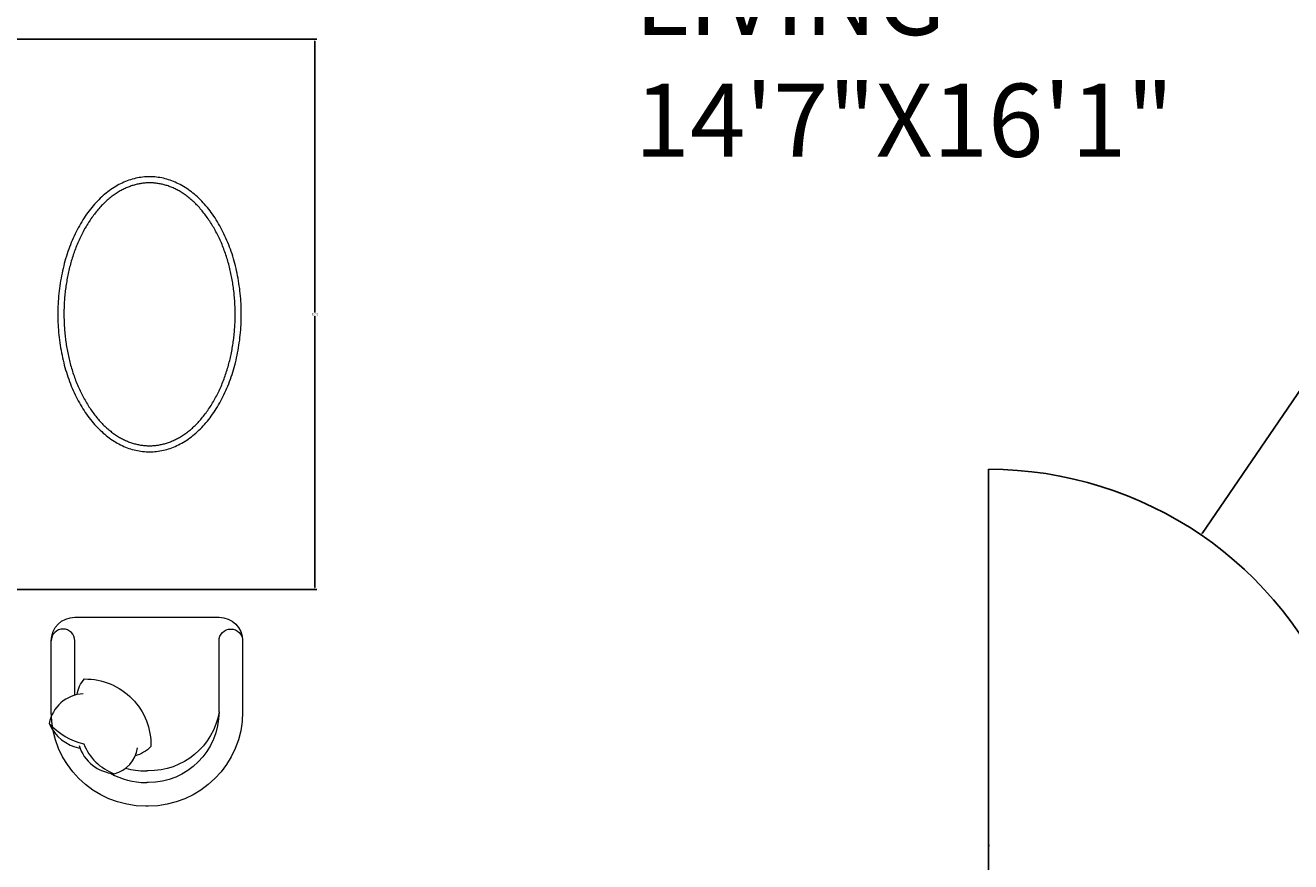
# Model space of a CAD drawing. Units: inches. Extents: x 1676 to 2199, y 1657 to 2783.
# Tile 3 of 10: x 1786 to 1907, y 1905 to 1985. Entities that reach past the tile are written whole.
import ezdxf

# ---------------------------------------------------------------- set-up
doc = ezdxf.new("R2010")
doc.units = ezdxf.units.IN
for name, color, linetype, lineweight in [('A-ANNO-DIMS', 2, 'Continuous', 18), ('A-AREA-IDEN', 7, 'Continuous', 18), ('A-DOOR', 4, 'Continuous', 25), ('A-FURN', 8, 'Continuous', 13)]:
    doc.layers.add(name, color=color, linetype=linetype, lineweight=lineweight)
doc.styles.get("Standard").update_dxf_attribs({"font": 'arial.ttf'})
doc.dimstyles.get("Standard").update_dxf_attribs({"dimtxt": 0.18, "dimasz": 0.18, "dimexe": 0.18, "dimexo": 0.0625, "dimgap": 0.09, "dimtad": 0, "dimtih": 1, "dimtoh": 1, "dimdec": 4, "dimzin": 0, "dimdsep": 46, "dimtxsty": 'Standard', "dimcen": 0.09, "dimadec": 0, "dimazin": 0, "dimtfac": 1, "dimtdec": 4, "dimtofl": 0, "dimtmove": 0, "dimatfit": 3, "dimfxl": 1, "dimtolj": 1, "dimtzin": 0, "dimarcsym": 0})

# ---------------------------------------------------------------- blocks, each defined once
blk = doc.blocks.new('*D56')
at = {"layer": 'A-ANNO-DIMS', "color": 0, "lineweight": -2, "transparency": 16777216}
for p, q in [((1781.71, 1983.79), (1813.98, 1983.79)), ((1813.8, 1983.61), (1813.8, 1957.62)), ((1813.8, 1931.26), (1813.8, 1957.25)), ((1781.71, 1931.08), (1813.98, 1931.08))]:
    blk.add_line(p, q, dxfattribs=at)
at = {"layer": 'A-ANNO-DIMS', "color": 0, "transparency": 16777216}
for points in [[(1813.77, 1983.61), (1813.83, 1983.61), (1813.8, 1983.79)], [(1813.77, 1931.26), (1813.83, 1931.26), (1813.8, 1931.08)]]:
    blk.add_solid(points, dxfattribs=at)
at = {"layer": 'Defpoints', "color": 0, "transparency": 16777216}
for p in [(1781.65, 1983.79), (1781.65, 1931.08), (1813.8, 1931.08)]:
    blk.add_point(p, dxfattribs=at)
at = {"layer": 'A-ANNO-DIMS', "color": 0, "transparency": 16777216, "insert": (1813.8, 1957.43), "char_height": 0.18, "attachment_point": 5}
blk.add_mtext('\\A1;52.72', dxfattribs=at)
blk = doc.blocks.new('*D81')
at = {"layer": 'A-ANNO-DIMS', "color": 0, "lineweight": -2, "transparency": 16777216}
for p, q in [((1910.86, 1954.14), (1898.76, 1936.45)), ((1911.04, 1954.14), (1910.86, 1954.14)), ((1878.23, 1906.55), (1878.41, 1906.55)), ((1878.32, 1906.46), (1878.32, 1906.64))]:
    blk.add_line(p, q, dxfattribs=at)
at = {"layer": 'A-ANNO-DIMS', "color": 0, "transparency": 16777216}
blk.add_solid([(1898.73, 1936.46), (1898.78, 1936.43), (1898.66, 1936.3)], dxfattribs=at)
at = {"layer": 'Defpoints', "color": 0, "transparency": 16777216}
for p in [(1898.66, 1936.3), (1878.32, 1906.55)]:
    blk.add_point(p, dxfattribs=at)
at = {"layer": 'A-ANNO-DIMS', "color": 0, "transparency": 16777216, "insert": (1911.59, 1954.14), "char_height": 0.18, "attachment_point": 5}
blk.add_mtext('\\A1;R36.034', dxfattribs=at)

msp = doc.modelspace()

# ---------------------------------------------------------------- linework, layer by layer
at = {"layer": 'A-DOOR'}
msp.add_line((1878.3163, 1894.5871), (1878.3163, 1942.5871), dxfattribs=at)
msp.add_arc((1878.3163, 1906.5528), 36.0343, 21.266188, 90, dxfattribs=at)
at = {"layer": 'A-FURN', "ltscale": 0.03}
msp.add_lwpolyline([(1797.7122, 1928.4136), (1804.6154, 1928.4136, -0.41421356), (1806.8787, 1926.1503), (1806.8787, 1919.3603, -0.41421356), (1797.8254, 1910.307), (1797.7122, 1910.307), (1797.5991, 1910.307, -0.41421356), (1788.5457, 1919.3603), (1788.5457, 1926.1503, -0.41421356), (1790.8091, 1928.4136), (1797.7122, 1928.4136)], format="xyb", dxfattribs=at)
at = {"layer": 'A-FURN'}
for points in [[(1790.8091, 1920.947), (1790.8091, 1926.1503, 0.41421356), (1789.6774, 1927.282), (1789.6774, 1927.282, 0.41421356), (1788.5457, 1926.1503)], [(1804.6154, 1919.3602), (1804.6154, 1926.1503, -0.41421356), (1805.7471, 1927.282), (1805.7471, 1927.282, -0.41421356), (1806.8787, 1926.1503)], [(1791.0329, 1921.0014, -0.16554063), (1791.733, 1922.4967, -0.42598917), (1798.0887, 1916.0137, -0.12152332), (1796.58, 1915.1202, 7.11546429)], [(1791.6033, 1921.0704, 0.35677236), (1788.3606, 1918.2179, 0.24954205), (1791.2988, 1915.8672, -9.61688035)], [(1804.6154, 1919.3603, -0.37271891), (1797.8254, 1913.702), (1797.7122, 1913.702)], [(1804.6154, 1919.3603, -0.41421356), (1797.8254, 1912.5703), (1797.7122, 1912.5703)], [(1788.3606, 1918.2179, 0.14772988), (1791.6682, 1916.273, 0.21334276), (1794.5866, 1913.4205, 0.17866181)], [(1791.2112, 1916.118, 0.30666349), (1794.5866, 1913.4205, 0.30632997), (1796.7916, 1915.8841, -0.87284716)], [(1795.6696, 1913.9458, 0.07238424), (1797.5991, 1913.702), (1797.7122, 1913.702)], [(1794.2286, 1913.4659, 0.13059149), (1797.5991, 1912.5703), (1797.7122, 1912.5703)]]:
    msp.add_lwpolyline(points, format="xyb", dxfattribs=at)
at = {"layer": 'A-FURN', "ltscale": 0.03}
msp.add_polyline3d([(1797.9632, 1970.6124, 0), (1797.797, 1970.61, 0), (1797.6308, 1970.603, 0), (1797.4647, 1970.5912, 0), (1797.2988, 1970.5746, 0), (1797.1331, 1970.5534, 0), (1796.9677, 1970.5275, 0), (1796.8027, 1970.4969, 0), (1796.6381, 1970.4616, 0), (1796.474, 1970.4217, 0), (1796.3104, 1970.3771, 0), (1796.1474, 1970.3278, 0), (1795.9851, 1970.274, 0), (1795.8234, 1970.2155, 0), (1795.6625, 1970.1525, 0), (1795.5025, 1970.0849, 0), (1795.3433, 1970.0128, 0), (1795.1851, 1969.9362, 0), (1795.0279, 1969.8551, 0), (1794.8717, 1969.7695, 0), (1794.7166, 1969.6796, 0), (1794.5627, 1969.5852, 0), (1794.41, 1969.4865, 0), (1794.2586, 1969.3835, 0), (1794.1085, 1969.2762, 0), (1793.9597, 1969.1646, 0), (1793.8125, 1969.0489, 0), (1793.6667, 1968.929, 0), (1793.5224, 1968.805, 0), (1793.3797, 1968.6769, 0), (1793.2387, 1968.5448, 0), (1793.0994, 1968.4087, 0), (1792.9618, 1968.2686, 0), (1792.826, 1968.1247, 0), (1792.692, 1967.977, 0), (1792.56, 1967.8255, 0), (1792.4298, 1967.6702, 0), (1792.3017, 1967.5113, 0), (1792.1755, 1967.3488, 0), (1792.0515, 1967.1827, 0), (1791.9296, 1967.0132, 0), (1791.8098, 1966.8402, 0), (1791.6922, 1966.6638, 0), (1791.5769, 1966.4842, 0), (1791.4638, 1966.3013, 0), (1791.3531, 1966.1152, 0), (1791.2448, 1965.926, 0), (1791.1389, 1965.7337, 0), (1791.0354, 1965.5385, 0), (1790.9343, 1965.3404, 0), (1790.8359, 1965.1395, 0), (1790.7399, 1964.9358, 0), (1790.6466, 1964.7294, 0), (1790.5558, 1964.5204, 0), (1790.4677, 1964.3089, 0), (1790.3823, 1964.0949, 0), (1790.2997, 1963.8785, 0), (1790.2197, 1963.6598, 0), (1790.1426, 1963.4389, 0), (1790.0682, 1963.2158, 0), (1789.9967, 1962.9906, 0), (1789.928, 1962.7635, 0), (1789.8622, 1962.5345, 0), (1789.7993, 1962.3036, 0), (1789.7393, 1962.071, 0), (1789.6823, 1961.8367, 0), (1789.6282, 1961.6008, 0), (1789.5771, 1961.3635, 0), (1789.529, 1961.1247, 0), (1789.484, 1960.8847, 0), (1789.442, 1960.6434, 0), (1789.403, 1960.4009, 0), (1789.3671, 1960.1574, 0), (1789.3343, 1959.9129, 0), (1789.3045, 1959.6675, 0), (1789.2779, 1959.4213, 0), (1789.2544, 1959.1744, 0), (1789.234, 1958.9269, 0), (1789.2167, 1958.6788, 0), (1789.2026, 1958.4303, 0), (1789.1916, 1958.1815, 0), (1789.1837, 1957.9323, 0), (1789.179, 1957.683, 0), (1789.1774, 1957.4336, 0), (1789.179, 1957.1842, 0), (1789.1837, 1956.9349, 0), (1789.1916, 1956.6858, 0), (1789.2026, 1956.4369, 0), (1789.2167, 1956.1884, 0), (1789.234, 1955.9404, 0), (1789.2544, 1955.6928, 0), (1789.2779, 1955.4459, 0), (1789.3045, 1955.1998, 0), (1789.3343, 1954.9544, 0), (1789.3671, 1954.7099, 0), (1789.403, 1954.4663, 0), (1789.442, 1954.2239, 0), (1789.484, 1953.9826, 0), (1789.529, 1953.7425, 0), (1789.5771, 1953.5037, 0), (1789.6282, 1953.2664, 0), (1789.6823, 1953.0305, 0), (1789.7393, 1952.7963, 0), (1789.7993, 1952.5636, 0), (1789.8622, 1952.3328, 0), (1789.928, 1952.1037, 0), (1789.9967, 1951.8766, 0), (1790.0682, 1951.6514, 0), (1790.1426, 1951.4284, 0), (1790.2197, 1951.2074, 0), (1790.2997, 1950.9888, 0), (1790.3823, 1950.7724, 0), (1790.4677, 1950.5584, 0), (1790.5558, 1950.3468, 0), (1790.6466, 1950.1378, 0), (1790.7399, 1949.9314, 0), (1790.8359, 1949.7277, 0), (1790.9343, 1949.5268, 0), (1791.0354, 1949.3287, 0), (1791.1389, 1949.1335, 0), (1791.2448, 1948.9413, 0), (1791.3531, 1948.7521, 0), (1791.4638, 1948.566, 0), (1791.5769, 1948.3831, 0), (1791.6922, 1948.2034, 0), (1791.8098, 1948.0271, 0), (1791.9296, 1947.8541, 0), (1792.0515, 1947.6845, 0), (1792.1755, 1947.5184, 0), (1792.3017, 1947.3559, 0), (1792.4298, 1947.197, 0), (1792.56, 1947.0418, 0), (1792.692, 1946.8903, 0), (1792.826, 1946.7425, 0), (1792.9618, 1946.5986, 0), (1793.0994, 1946.4586, 0), (1793.2387, 1946.3225, 0), (1793.3797, 1946.1904, 0), (1793.5224, 1946.0623, 0), (1793.6667, 1945.9382, 0), (1793.8125, 1945.8183, 0), (1793.9597, 1945.7026, 0), (1794.1085, 1945.591, 0), (1794.2586, 1945.4837, 0), (1794.41, 1945.3807, 0), (1794.5627, 1945.282, 0), (1794.7166, 1945.1877, 0), (1794.8717, 1945.0977, 0), (1795.0279, 1945.0122, 0), (1795.1851, 1944.9311, 0), (1795.3433, 1944.8544, 0), (1795.5025, 1944.7823, 0), (1795.6625, 1944.7147, 0), (1795.8234, 1944.6517, 0), (1795.9851, 1944.5932, 0), (1796.1474, 1944.5394, 0), (1796.3104, 1944.4902, 0), (1796.474, 1944.4456, 0), (1796.6381, 1944.4056, 0), (1796.8027, 1944.3703, 0), (1796.9677, 1944.3397, 0), (1797.1331, 1944.3138, 0), (1797.2988, 1944.2926, 0), (1797.4647, 1944.2761, 0), (1797.6308, 1944.2643, 0), (1797.797, 1944.2572, 0), (1797.9632, 1944.2548, 0), (1798.1295, 1944.2572, 0), (1798.2957, 1944.2643, 0), (1798.4618, 1944.2761, 0), (1798.6277, 1944.2926, 0), (1798.7934, 1944.3138, 0), (1798.9588, 1944.3397, 0), (1799.1238, 1944.3703, 0), (1799.2884, 1944.4056, 0), (1799.4525, 1944.4456, 0), (1799.6161, 1944.4902, 0), (1799.7791, 1944.5394, 0), (1799.9414, 1944.5932, 0), (1800.1031, 1944.6517, 0), (1800.2639, 1944.7147, 0), (1800.424, 1944.7823, 0), (1800.5832, 1944.8544, 0), (1800.7414, 1944.9311, 0), (1800.8986, 1945.0122, 0), (1801.0548, 1945.0977, 0), (1801.2099, 1945.1877, 0), (1801.3638, 1945.282, 0), (1801.5165, 1945.3807, 0), (1801.6679, 1945.4837, 0), (1801.818, 1945.591, 0), (1801.9667, 1945.7026, 0), (1802.114, 1945.8183, 0), (1802.2598, 1945.9382, 0), (1802.4041, 1946.0623, 0), (1802.5467, 1946.1904, 0), (1802.6878, 1946.3225, 0), (1802.8271, 1946.4586, 0), (1802.9647, 1946.5986, 0), (1803.1005, 1946.7425, 0), (1803.2345, 1946.8903, 0), (1803.3665, 1947.0418, 0), (1803.4967, 1947.197, 0), (1803.6248, 1947.3559, 0), (1803.7509, 1947.5184, 0), (1803.875, 1947.6845, 0), (1803.9969, 1947.8541, 0), (1804.1167, 1948.0271, 0), (1804.2343, 1948.2034, 0), (1804.3496, 1948.3831, 0), (1804.4627, 1948.566, 0), (1804.5734, 1948.7521, 0), (1804.6817, 1948.9413, 0), (1804.7876, 1949.1335, 0), (1804.8911, 1949.3287, 0), (1804.9921, 1949.5268, 0), (1805.0906, 1949.7277, 0), (1805.1866, 1949.9314, 0), (1805.2799, 1950.1378, 0), (1805.3707, 1950.3468, 0), (1805.4588, 1950.5584, 0), (1805.5442, 1950.7724, 0), (1805.6268, 1950.9888, 0), (1805.7068, 1951.2074, 0), (1805.7839, 1951.4284, 0), (1805.8583, 1951.6514, 0), (1805.9298, 1951.8766, 0), (1805.9985, 1952.1037, 0), (1806.0643, 1952.3328, 0), (1806.1272, 1952.5636, 0), (1806.1872, 1952.7963, 0), (1806.2442, 1953.0305, 0), (1806.2983, 1953.2664, 0), (1806.3494, 1953.5037, 0), (1806.3975, 1953.7425, 0), (1806.4425, 1953.9826, 0), (1806.4845, 1954.2239, 0), (1806.5235, 1954.4663, 0), (1806.5594, 1954.7099, 0), (1806.5922, 1954.9544, 0), (1806.622, 1955.1998, 0), (1806.6486, 1955.4459, 0), (1806.6721, 1955.6928, 0), (1806.6925, 1955.9404, 0), (1806.7098, 1956.1884, 0), (1806.7239, 1956.4369, 0), (1806.7349, 1956.6858, 0), (1806.7428, 1956.9349, 0), (1806.7475, 1957.1842, 0), (1806.7491, 1957.4336, 0), (1806.7475, 1957.683, 0), (1806.7428, 1957.9323, 0), (1806.7349, 1958.1815, 0), (1806.7239, 1958.4303, 0), (1806.7098, 1958.6788, 0), (1806.6925, 1958.9269, 0), (1806.6721, 1959.1744, 0), (1806.6486, 1959.4213, 0), (1806.622, 1959.6675, 0), (1806.5922, 1959.9129, 0), (1806.5594, 1960.1574, 0), (1806.5235, 1960.4009, 0), (1806.4845, 1960.6434, 0), (1806.4425, 1960.8847, 0), (1806.3975, 1961.1247, 0), (1806.3494, 1961.3635, 0), (1806.2983, 1961.6008, 0), (1806.2442, 1961.8367, 0), (1806.1872, 1962.071, 0), (1806.1272, 1962.3036, 0), (1806.0643, 1962.5345, 0), (1805.9985, 1962.7635, 0), (1805.9298, 1962.9906, 0), (1805.8583, 1963.2158, 0), (1805.7839, 1963.4389, 0), (1805.7068, 1963.6598, 0), (1805.6268, 1963.8785, 0), (1805.5442, 1964.0949, 0), (1805.4588, 1964.3089, 0), (1805.3707, 1964.5204, 0), (1805.2799, 1964.7294, 0), (1805.1866, 1964.9358, 0), (1805.0906, 1965.1395, 0), (1804.9921, 1965.3404, 0), (1804.8911, 1965.5385, 0), (1804.7876, 1965.7337, 0), (1804.6817, 1965.926, 0), (1804.5734, 1966.1152, 0), (1804.4627, 1966.3013, 0), (1804.3496, 1966.4842, 0), (1804.2343, 1966.6638, 0), (1804.1167, 1966.8402, 0), (1803.9969, 1967.0132, 0), (1803.875, 1967.1827, 0), (1803.7509, 1967.3488, 0), (1803.6248, 1967.5113, 0), (1803.4967, 1967.6702, 0), (1803.3665, 1967.8255, 0), (1803.2345, 1967.977, 0), (1803.1005, 1968.1247, 0), (1802.9647, 1968.2686, 0), (1802.8271, 1968.4087, 0), (1802.6878, 1968.5448, 0), (1802.5467, 1968.6769, 0), (1802.4041, 1968.805, 0), (1802.2598, 1968.929, 0), (1802.114, 1969.0489, 0), (1801.9667, 1969.1646, 0), (1801.818, 1969.2762, 0), (1801.6679, 1969.3835, 0), (1801.5165, 1969.4865, 0), (1801.3638, 1969.5852, 0), (1801.2099, 1969.6796, 0), (1801.0548, 1969.7695, 0), (1800.8986, 1969.8551, 0), (1800.7414, 1969.9362, 0), (1800.5832, 1970.0128, 0), (1800.424, 1970.0849, 0), (1800.2639, 1970.1525, 0), (1800.1031, 1970.2155, 0), (1799.9414, 1970.274, 0), (1799.7791, 1970.3278, 0), (1799.6161, 1970.3771, 0), (1799.4525, 1970.4217, 0), (1799.2884, 1970.4616, 0), (1799.1238, 1970.4969, 0), (1798.9588, 1970.5275, 0), (1798.7934, 1970.5534, 0), (1798.6277, 1970.5746, 0), (1798.4618, 1970.5912, 0), (1798.2957, 1970.603, 0), (1798.1295, 1970.61, 0), (1797.9632, 1970.6124, 0)], dxfattribs=at)
at = {"layer": 'A-FURN'}
msp.add_polyline3d([(1797.9632, 1970.0267, 0), (1797.8734, 1970.0259, 0), (1797.7831, 1970.0236, 0), (1797.6925, 1970.0197, 0), (1797.6014, 1970.0142, 0), (1797.51, 1970.0071, 0), (1797.4182, 1969.9984, 0), (1797.326, 1969.9881, 0), (1797.2335, 1969.976, 0), (1797.1407, 1969.9623, 0), (1797.0476, 1969.9469, 0), (1796.9541, 1969.9297, 0), (1796.8604, 1969.9108, 0), (1796.7664, 1969.8901, 0), (1796.6721, 1969.8676, 0), (1796.5776, 1969.8433, 0), (1796.4829, 1969.8172, 0), (1796.3879, 1969.7892, 0), (1796.2927, 1969.7594, 0), (1796.1973, 1969.7276, 0), (1796.1017, 1969.6939, 0), (1796.0059, 1969.6583, 0), (1795.91, 1969.6208, 0), (1795.814, 1969.5812, 0), (1795.7179, 1969.5396, 0), (1795.6217, 1969.4961, 0), (1795.5255, 1969.4506, 0), (1795.4293, 1969.403, 0), (1795.3331, 1969.3535, 0), (1795.2369, 1969.3019, 0), (1795.1409, 1969.2484, 0), (1795.0449, 1969.1928, 0), (1794.9491, 1969.1352, 0), (1794.8535, 1969.0756, 0), (1794.758, 1969.014, 0), (1794.6628, 1968.9503, 0), (1794.5678, 1968.8847, 0), (1794.4732, 1968.817, 0), (1794.3788, 1968.7473, 0), (1794.2847, 1968.6755, 0), (1794.1911, 1968.6017, 0), (1794.0978, 1968.5259, 0), (1794.005, 1968.448, 0), (1793.9126, 1968.3679, 0), (1793.8206, 1968.2856, 0), (1793.7292, 1968.2012, 0), (1793.6383, 1968.1146, 0), (1793.5479, 1968.026, 0), (1793.4581, 1967.9352, 0), (1793.3688, 1967.8425, 0), (1793.2802, 1967.7477, 0), (1793.1923, 1967.651, 0), (1793.1049, 1967.5524, 0), (1793.0183, 1967.4518, 0), (1792.9324, 1967.3493, 0), (1792.8472, 1967.245, 0), (1792.7628, 1967.1389, 0), (1792.6791, 1967.031, 0), (1792.5963, 1966.9213, 0), (1792.5143, 1966.8099, 0), (1792.4331, 1966.6968, 0), (1792.3528, 1966.582, 0), (1792.2735, 1966.4656, 0), (1792.195, 1966.3476, 0), (1792.1175, 1966.228, 0), (1792.041, 1966.1069, 0), (1791.9655, 1965.9843, 0), (1791.8909, 1965.8601, 0), (1791.8175, 1965.7346, 0), (1791.7451, 1965.6076, 0), (1791.6738, 1965.4792, 0), (1791.6036, 1965.3494, 0), (1791.5346, 1965.2184, 0), (1791.4667, 1965.086, 0), (1791.4, 1964.9523, 0), (1791.3345, 1964.8175, 0), (1791.2703, 1964.6814, 0), (1791.2073, 1964.5441, 0), (1791.1456, 1964.4057, 0), (1791.0853, 1964.2662, 0), (1791.0262, 1964.1256, 0), (1790.9686, 1963.9839, 0), (1790.9123, 1963.8412, 0), (1790.8574, 1963.6976, 0), (1790.8039, 1963.5531, 0), (1790.7518, 1963.4082, 0), (1790.7012, 1963.263, 0), (1790.652, 1963.1173, 0), (1790.6041, 1962.9713, 0), (1790.5577, 1962.8249, 0), (1790.5126, 1962.6782, 0), (1790.469, 1962.5311, 0), (1790.4267, 1962.3837, 0), (1790.3858, 1962.2359, 0), (1790.3462, 1962.0879, 0), (1790.308, 1961.9395, 0), (1790.2712, 1961.7908, 0), (1790.2356, 1961.6419, 0), (1790.2015, 1961.4926, 0), (1790.1686, 1961.3431, 0), (1790.1371, 1961.1934, 0), (1790.107, 1961.0434, 0), (1790.0781, 1960.8932, 0), (1790.0505, 1960.7427, 0), (1790.0243, 1960.592, 0), (1789.9993, 1960.4411, 0), (1789.9756, 1960.2901, 0), (1789.9533, 1960.1388, 0), (1789.9322, 1959.9873, 0), (1789.9123, 1959.8357, 0), (1789.8938, 1959.684, 0), (1789.8765, 1959.532, 0), (1789.8604, 1959.38, 0), (1789.8456, 1959.2278, 0), (1789.832, 1959.0755, 0), (1789.8197, 1958.9231, 0), (1789.8086, 1958.7706, 0), (1789.7988, 1958.618, 0), (1789.7901, 1958.4654, 0), (1789.7827, 1958.3126, 0), (1789.7764, 1958.1598, 0), (1789.7714, 1958.007, 0), (1789.7676, 1957.8541, 0), (1789.7649, 1957.7012, 0), (1789.7635, 1957.5483, 0), (1789.7632, 1957.3954, 0), (1789.764, 1957.2425, 0), (1789.7661, 1957.0896, 0), (1789.7693, 1956.9367, 0), (1789.7738, 1956.7838, 0), (1789.7794, 1956.631, 0), (1789.7862, 1956.4782, 0), (1789.7943, 1956.3255, 0), (1789.8035, 1956.1729, 0), (1789.814, 1956.0204, 0), (1789.8257, 1955.8679, 0), (1789.8387, 1955.7156, 0), (1789.8529, 1955.5633, 0), (1789.8683, 1955.4112, 0), (1789.885, 1955.2592, 0), (1789.9029, 1955.1074, 0), (1789.9221, 1954.9557, 0), (1789.9426, 1954.8042, 0), (1789.9643, 1954.6528, 0), (1789.9873, 1954.5016, 0), (1790.0116, 1954.3506, 0), (1790.0372, 1954.1999, 0), (1790.0641, 1954.0493, 0), (1790.0924, 1953.8989, 0), (1790.1219, 1953.7488, 0), (1790.1527, 1953.5989, 0), (1790.1849, 1953.4493, 0), (1790.2184, 1953.2999, 0), (1790.2532, 1953.1509, 0), (1790.2894, 1953.002, 0), (1790.3269, 1952.8535, 0), (1790.3658, 1952.7053, 0), (1790.4061, 1952.5574, 0), (1790.4477, 1952.4098, 0), (1790.4906, 1952.2625, 0), (1790.535, 1952.1156, 0), (1790.5807, 1951.9691, 0), (1790.6279, 1951.8229, 0), (1790.6764, 1951.677, 0), (1790.7263, 1951.5316, 0), (1790.7777, 1951.3865, 0), (1790.8304, 1951.2419, 0), (1790.8846, 1951.0977, 0), (1790.9402, 1950.9545, 0), (1790.9972, 1950.8124, 0), (1791.0556, 1950.6712, 0), (1791.1153, 1950.5312, 0), (1791.1763, 1950.3922, 0), (1791.2387, 1950.2544, 0), (1791.3023, 1950.1177, 0), (1791.3671, 1949.9822, 0), (1791.4332, 1949.8479, 0), (1791.5005, 1949.7149, 0), (1791.5689, 1949.5832, 0), (1791.6386, 1949.4528, 0), (1791.7093, 1949.3237, 0), (1791.7811, 1949.196, 0), (1791.8541, 1949.0697, 0), (1791.9281, 1948.9449, 0), (1792.0031, 1948.8215, 0), (1792.0791, 1948.6996, 0), (1792.1561, 1948.5792, 0), (1792.2341, 1948.4604, 0), (1792.313, 1948.3432, 0), (1792.3929, 1948.2276, 0), (1792.4736, 1948.1137, 0), (1792.5552, 1948.0014, 0), (1792.6376, 1947.8909, 0), (1792.7209, 1947.7821, 0), (1792.8049, 1947.6751, 0), (1792.8897, 1947.5698, 0), (1792.9753, 1947.4665, 0), (1793.0615, 1947.3649, 0), (1793.1485, 1947.2653, 0), (1793.2362, 1947.1676, 0), (1793.3245, 1947.0719, 0), (1793.4134, 1946.9781, 0), (1793.5029, 1946.8864, 0), (1793.593, 1946.7967, 0), (1793.6837, 1946.7091, 0), (1793.7748, 1946.6236, 0), (1793.8665, 1946.5402, 0), (1793.9587, 1946.4591, 0), (1794.0513, 1946.3801, 0), (1794.1444, 1946.3032, 0), (1794.2379, 1946.2284, 0), (1794.3317, 1946.1556, 0), (1794.4259, 1946.0849, 0), (1794.5205, 1946.0162, 0), (1794.6153, 1945.9495, 0), (1794.7104, 1945.8848, 0), (1794.8057, 1945.8222, 0), (1794.9013, 1945.7616, 0), (1794.997, 1945.703, 0), (1795.0929, 1945.6464, 0), (1795.1889, 1945.5918, 0), (1795.285, 1945.5393, 0), (1795.3812, 1945.4887, 0), (1795.4774, 1945.4402, 0), (1795.5736, 1945.3937, 0), (1795.6698, 1945.3491, 0), (1795.7659, 1945.3066, 0), (1795.862, 1945.266, 0), (1795.958, 1945.2274, 0), (1796.0538, 1945.1909, 0), (1796.1495, 1945.1562, 0), (1796.245, 1945.1235, 0), (1796.3403, 1945.0927, 0), (1796.4354, 1945.0638, 0), (1796.5303, 1945.0368, 0), (1796.6249, 1945.0115, 0), (1796.7193, 1944.9882, 0), (1796.8134, 1944.9666, 0), (1796.9073, 1944.9468, 0), (1797.0009, 1944.9287, 0), (1797.0942, 1944.9124, 0), (1797.1871, 1944.8979, 0), (1797.2798, 1944.885, 0), (1797.3721, 1944.8738, 0), (1797.4641, 1944.8642, 0), (1797.5557, 1944.8564, 0), (1797.647, 1944.8501, 0), (1797.7378, 1944.8454, 0), (1797.8283, 1944.8423, 0), (1797.9184, 1944.8408, 0), (1798.0081, 1944.8408, 0), (1798.0982, 1944.8423, 0), (1798.1887, 1944.8454, 0), (1798.2795, 1944.8501, 0), (1798.3708, 1944.8564, 0), (1798.4624, 1944.8642, 0), (1798.5544, 1944.8738, 0), (1798.6467, 1944.885, 0), (1798.7393, 1944.8979, 0), (1798.8323, 1944.9124, 0), (1798.9256, 1944.9287, 0), (1799.0192, 1944.9468, 0), (1799.1131, 1944.9666, 0), (1799.2072, 1944.9882, 0), (1799.3016, 1945.0115, 0), (1799.3962, 1945.0368, 0), (1799.4911, 1945.0638, 0), (1799.5862, 1945.0927, 0), (1799.6815, 1945.1235, 0), (1799.777, 1945.1562, 0), (1799.8727, 1945.1909, 0), (1799.9685, 1945.2274, 0), (1800.0645, 1945.266, 0), (1800.1605, 1945.3066, 0), (1800.2567, 1945.3491, 0), (1800.3529, 1945.3937, 0), (1800.4491, 1945.4402, 0), (1800.5453, 1945.4887, 0), (1800.6415, 1945.5393, 0), (1800.7376, 1945.5918, 0), (1800.8336, 1945.6464, 0), (1800.9295, 1945.703, 0), (1801.0252, 1945.7616, 0), (1801.1208, 1945.8222, 0), (1801.2161, 1945.8848, 0), (1801.3112, 1945.9495, 0), (1801.406, 1946.0162, 0), (1801.5006, 1946.0849, 0), (1801.5948, 1946.1556, 0), (1801.6886, 1946.2284, 0), (1801.7821, 1946.3032, 0), (1801.8752, 1946.3801, 0), (1801.9678, 1946.4591, 0), (1802.06, 1946.5402, 0), (1802.1516, 1946.6236, 0), (1802.2428, 1946.7091, 0), (1802.3335, 1946.7967, 0), (1802.4236, 1946.8864, 0), (1802.5131, 1946.9781, 0), (1802.602, 1947.0719, 0), (1802.6903, 1947.1676, 0), (1802.778, 1947.2653, 0), (1802.865, 1947.3649, 0), (1802.9512, 1947.4665, 0), (1803.0368, 1947.5698, 0), (1803.1216, 1947.6751, 0), (1803.2056, 1947.7821, 0), (1803.2889, 1947.8909, 0), (1803.3713, 1948.0014, 0), (1803.4529, 1948.1137, 0), (1803.5336, 1948.2276, 0), (1803.6135, 1948.3432, 0), (1803.6924, 1948.4604, 0), (1803.7704, 1948.5792, 0), (1803.8474, 1948.6996, 0), (1803.9234, 1948.8215, 0), (1803.9984, 1948.9449, 0), (1804.0724, 1949.0697, 0), (1804.1453, 1949.196, 0), (1804.2172, 1949.3237, 0), (1804.2879, 1949.4528, 0), (1804.3576, 1949.5832, 0), (1804.426, 1949.7149, 0), (1804.4933, 1949.8479, 0), (1804.5594, 1949.9822, 0), (1804.6242, 1950.1177, 0), (1804.6878, 1950.2544, 0), (1804.7502, 1950.3922, 0), (1804.8112, 1950.5312, 0), (1804.8709, 1950.6712, 0), (1804.9293, 1950.8124, 0), (1804.9863, 1950.9545, 0), (1805.0419, 1951.0977, 0), (1805.096, 1951.2419, 0), (1805.1488, 1951.3865, 0), (1805.2001, 1951.5316, 0), (1805.2501, 1951.677, 0), (1805.2986, 1951.8229, 0), (1805.3458, 1951.9691, 0), (1805.3915, 1952.1156, 0), (1805.4359, 1952.2625, 0), (1805.4788, 1952.4098, 0), (1805.5204, 1952.5574, 0), (1805.5607, 1952.7053, 0), (1805.5996, 1952.8535, 0), (1805.6371, 1953.002, 0), (1805.6733, 1953.1509, 0), (1805.7081, 1953.2999, 0), (1805.7416, 1953.4493, 0), (1805.7738, 1953.5989, 0), (1805.8046, 1953.7488, 0), (1805.8341, 1953.8989, 0), (1805.8623, 1954.0493, 0), (1805.8893, 1954.1999, 0), (1805.9149, 1954.3506, 0), (1805.9392, 1954.5016, 0), (1805.9622, 1954.6528, 0), (1805.9839, 1954.8042, 0), (1806.0044, 1954.9557, 0), (1806.0236, 1955.1074, 0), (1806.0415, 1955.2592, 0), (1806.0582, 1955.4112, 0), (1806.0736, 1955.5633, 0), (1806.0878, 1955.7156, 0), (1806.1008, 1955.8679, 0), (1806.1125, 1956.0204, 0), (1806.1229, 1956.1729, 0), (1806.1322, 1956.3255, 0), (1806.1403, 1956.4782, 0), (1806.1471, 1956.631, 0), (1806.1527, 1956.7838, 0), (1806.1572, 1956.9367, 0), (1806.1604, 1957.0896, 0), (1806.1625, 1957.2425, 0), (1806.1633, 1957.3954, 0), (1806.163, 1957.5483, 0), (1806.1616, 1957.7012, 0), (1806.1589, 1957.8541, 0), (1806.1551, 1958.007, 0), (1806.1501, 1958.1598, 0), (1806.1438, 1958.3126, 0), (1806.1364, 1958.4654, 0), (1806.1277, 1958.618, 0), (1806.1179, 1958.7706, 0), (1806.1068, 1958.9231, 0), (1806.0944, 1959.0755, 0), (1806.0809, 1959.2278, 0), (1806.0661, 1959.38, 0), (1806.05, 1959.532, 0), (1806.0327, 1959.684, 0), (1806.0142, 1959.8357, 0), (1805.9943, 1959.9873, 0), (1805.9732, 1960.1388, 0), (1805.9508, 1960.2901, 0), (1805.9272, 1960.4411, 0), (1805.9022, 1960.592, 0), (1805.876, 1960.7427, 0), (1805.8484, 1960.8932, 0), (1805.8195, 1961.0434, 0), (1805.7894, 1961.1934, 0), (1805.7578, 1961.3431, 0), (1805.725, 1961.4926, 0), (1805.6908, 1961.6419, 0), (1805.6553, 1961.7908, 0), (1805.6185, 1961.9395, 0), (1805.5803, 1962.0879, 0), (1805.5407, 1962.2359, 0), (1805.4998, 1962.3837, 0), (1805.4575, 1962.5311, 0), (1805.4138, 1962.6782, 0), (1805.3688, 1962.8249, 0), (1805.3224, 1962.9713, 0), (1805.2745, 1963.1173, 0), (1805.2253, 1963.263, 0), (1805.1747, 1963.4082, 0), (1805.1226, 1963.5531, 0), (1805.0691, 1963.6976, 0), (1805.0142, 1963.8412, 0), (1804.9579, 1963.9839, 0), (1804.9003, 1964.1256, 0), (1804.8412, 1964.2662, 0), (1804.7808, 1964.4057, 0), (1804.7192, 1964.5441, 0), (1804.6562, 1964.6814, 0), (1804.592, 1964.8175, 0), (1804.5265, 1964.9523, 0), (1804.4598, 1965.086, 0), (1804.3919, 1965.2184, 0), (1804.3229, 1965.3494, 0), (1804.2527, 1965.4792, 0), (1804.1814, 1965.6076, 0), (1804.109, 1965.7346, 0), (1804.0356, 1965.8601, 0), (1803.961, 1965.9843, 0), (1803.8855, 1966.1069, 0), (1803.809, 1966.228, 0), (1803.7315, 1966.3476, 0), (1803.653, 1966.4656, 0), (1803.5736, 1966.582, 0), (1803.4934, 1966.6968, 0), (1803.4122, 1966.8099, 0), (1803.3302, 1966.9213, 0), (1803.2474, 1967.031, 0), (1803.1637, 1967.1389, 0), (1803.0793, 1967.245, 0), (1802.9941, 1967.3493, 0), (1802.9082, 1967.4518, 0), (1802.8216, 1967.5524, 0), (1802.7342, 1967.651, 0), (1802.6463, 1967.7477, 0), (1802.5576, 1967.8425, 0), (1802.4684, 1967.9352, 0), (1802.3786, 1968.026, 0), (1802.2882, 1968.1146, 0), (1802.1973, 1968.2012, 0), (1802.1059, 1968.2856, 0), (1802.0139, 1968.3679, 0), (1801.9215, 1968.448, 0), (1801.8287, 1968.5259, 0), (1801.7354, 1968.6017, 0), (1801.6417, 1968.6755, 0), (1801.5477, 1968.7473, 0), (1801.4533, 1968.817, 0), (1801.3586, 1968.8847, 0), (1801.2637, 1968.9503, 0), (1801.1685, 1969.014, 0), (1801.073, 1969.0756, 0), (1800.9774, 1969.1352, 0), (1800.8816, 1969.1928, 0), (1800.7856, 1969.2484, 0), (1800.6896, 1969.3019, 0), (1800.5934, 1969.3535, 0), (1800.4972, 1969.403, 0), (1800.401, 1969.4506, 0), (1800.3048, 1969.4961, 0), (1800.2086, 1969.5396, 0), (1800.1125, 1969.5812, 0), (1800.0165, 1969.6208, 0), (1799.9206, 1969.6583, 0), (1799.8248, 1969.6939, 0), (1799.7292, 1969.7276, 0), (1799.6338, 1969.7594, 0), (1799.5386, 1969.7892, 0), (1799.4436, 1969.8172, 0), (1799.3489, 1969.8433, 0), (1799.2544, 1969.8676, 0), (1799.1601, 1969.8901, 0), (1799.0661, 1969.9108, 0), (1798.9724, 1969.9297, 0), (1798.8789, 1969.9469, 0), (1798.7858, 1969.9623, 0), (1798.693, 1969.976, 0), (1798.6005, 1969.9881, 0), (1798.5083, 1969.9984, 0), (1798.4165, 1970.0071, 0), (1798.3251, 1970.0142, 0), (1798.234, 1970.0197, 0), (1798.1434, 1970.0236, 0), (1798.0531, 1970.0259, 0), (1797.9632, 1970.0267, 0)], dxfattribs=at)

# ---------------------------------------------------------------- texts
at = {"layer": 'A-AREA-IDEN', "insert": (1844.4148, 1991.1927), "char_height": 7, "attachment_point": 1}
msp.add_mtext_dynamic_manual_height_columns('LIVING \\P14\'7"X16\'1"', width=86.067539, gutter_width=12.5, heights=[0], dxfattribs=at)

# ---------------------------------------------------------------- dimensions: what is measured, and where the dimension line sits
at = {"layer": 'A-ANNO-DIMS'}
dim = msp.add_linear_dim(base=(1813.7967, 1931.0761), p1=(1781.6467, 1983.7912), p2=(1781.6467, 1931.0761), angle=270, dimstyle='Standard', override={"dimdec": 2, "dimlfac": 1, "dimrnd": 0, "dimzin": 0, "dimdsep": 46, "dimlunit": 2}, dxfattribs=at)
dim.commit()
dim.dimension.update_dxf_attribs({"geometry": '*D56', "text_midpoint": (1813.7967, 1957.4336)})
dim = msp.add_radius_dim(center=(1878.3163, 1906.5528), mpoint=(1898.6571, 1936.2971), dimstyle='Standard', override={"dimdec": 3, "dimlfac": 1, "dimrnd": 0, "dimzin": 0, "dimdsep": 46, "dimlunit": 2}, dxfattribs=at)
dim.commit()
dim.dimension.update_dxf_attribs({"geometry": '*D81', "text_midpoint": (1911.5909, 1954.1437), "dimtype": 164})

doc.saveas('drawing.dxf')
